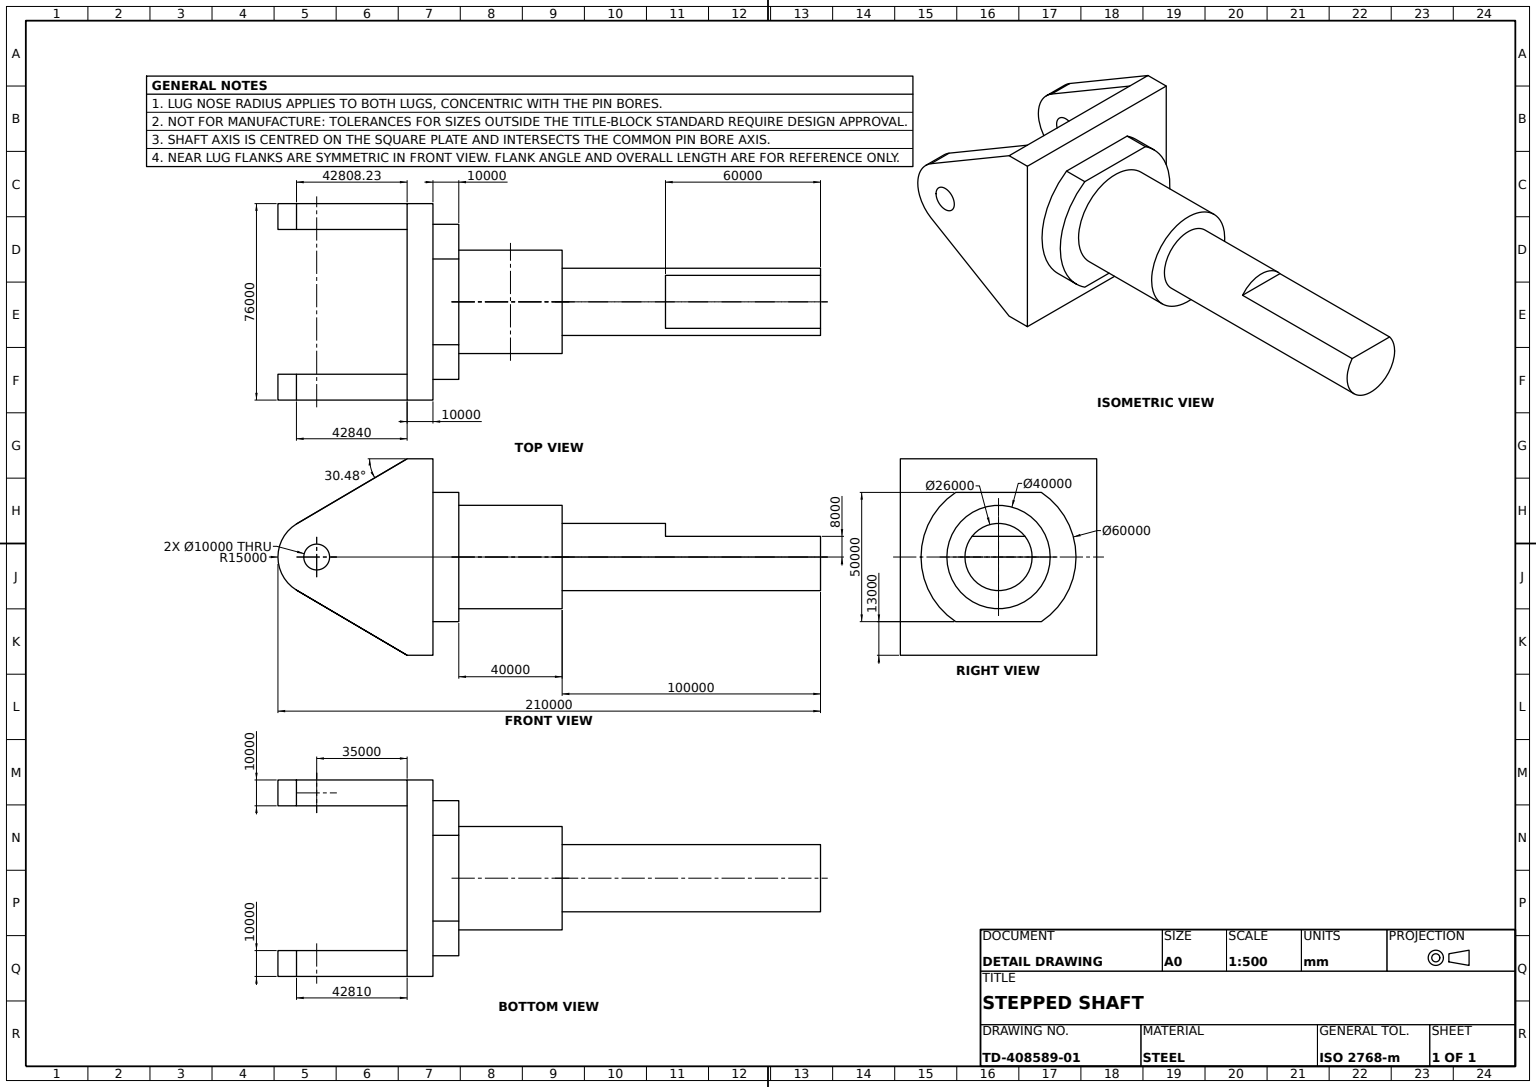
SolidWorks part; units mm, degrees
material "Plain Carbon Steel"
ref_plane "Front Plane" through (0, 0, 0) normal (0, 0, 1) x (1, 0, 0)
ref_plane "Top Plane" through (0, 0, 0) normal (0, 1, 0) x (1, 0, 0)
ref_plane "Right Plane" through (0, 0, 0) normal (1, 0, 0) x (0, 0, -1)
sketch "Base Plate Sketch" plane through (0, 0, 0) normal (0, 0, 1) x (1, 0, 0)
  line L5 (-38000, -38000) -> (38000, -38000)
  line L6 (-38000, -38000) -> (-38000, 38000)
  line L7 (-38000, 38000) -> (38000, 38000)
  line L8 (38000, -38000) -> (38000, 38000)
  line L9 (-38000, -38000) -> (38000, 38000) construction
  line L10 (-38000, 38000) -> (38000, -38000) construction
  point P0 (0, 0)
  dimension "D1" = 38000
extrude "Base Plate" add sketch "Base Plate Sketch" along normal blind 10000
sketch "Clevis Lug A Sketch" plane through (38000, 0, 0) normal (1, 0, 0) x (0, 0, -1)
  line L0 (0, 38000) -> (0, -38000)
  line L1 (0, 0) -> (35000, 0) construction
  line L2 (0, 38000) -> (42808.2335, 12807.4779)
  line L3 (0, -38000) -> (42810, -12806.4007)
  arc A0 (42810, -12806.4007) -> (42405.5538, 13044.4537) centre (35000, 0) ccw
  circle A1 centre (35000, 0) radius 5000
  dimension "D2" = 30000
  dimension "D3" = 10000
  dimension "D1" = 35000
  dimension "D4" = 42808.2335
  dimension "D5" = 42810
extrude "Clevis Lug A" add sketch "Clevis Lug A Sketch" against normal blind 10000
sketch "Clevis Lug B Sketch" plane through (-38000, 0, 0) normal (-1, 0, 0) x (0, 0, 1)
  line L0 (0, 38000) -> (0, -38000)
  line L1 (0, 38000) -> (-42840, 12788.0569)
  line L2 (0, -38000) -> (-42840, -12788.0569)
  circle A0 centre (-35000, 0) radius 5000
  arc A1 (-42840, 12788.0569) -> (-42840, -12788.0569) centre (-35000, 0) ccw
  dimension "D1" = 30000
  dimension "D2" = 10000
  dimension "D3" = 42840
  dimension "D4" = 42840
extrude "Clevis Lug B" add sketch "Clevis Lug B Sketch" against normal blind 10000
sketch "Collar Ø60 Sketch" plane through (0, 0, 10000) normal (0, 0, 1) x (1, 0, 0)
  circle A0 centre (0, 0) radius 30000
  dimension "D1" = 60000
extrude "Collar Ø60" add sketch "Collar Ø60 Sketch" along normal blind 10000
sketch "Hex Collar Cut Sketch" plane through (0, 0, 20000) normal (0, 0, 1) x (1, 0, 0)
  line L1 (-35000, 25000) -> (35000, 25000)
  line L2 (-35000, 25000) -> (-35000, -25000)
  line L3 (-35000, -25000) -> (35000, -25000)
  line L4 (35000, 25000) -> (35000, -25000)
  line L5 (-35000, 25000) -> (35000, -25000) construction
  line L6 (-35000, -25000) -> (35000, 25000) construction
  point P0 (0, 0)
  dimension "D1" = 50000
  dimension "D2" = 70000
extrude "Hex Collar Cut" cut sketch "Hex Collar Cut Sketch" against normal blind 10000 flip side to cut
sketch "Shaft Shoulder Ø40 Sketch" plane through (0, 0, 20000) normal (0, 0, 1) x (1, 0, 0)
  circle A0 centre (0, 0) radius 20000
  dimension "D1" = 40000
extrude "Shaft Shoulder Ø40" add sketch "Shaft Shoulder Ø40 Sketch" along normal blind 40000
sketch "Shaft Ø26 Sketch" plane through (0, 0, 60000) normal (0, 0, 1) x (1, 0, 0)
  circle A0 centre (0, 0) radius 13000
  dimension "D1" = 26000
extrude "Shaft Ø26" add sketch "Shaft Ø26 Sketch" along normal blind 100000
sketch "Shaft Flat Sketch" plane through (0, 0, 160000) normal (0, 0, 1) x (1, 0, 0)
  line L1 (-13341.8036, 8000) -> (13341.8036, 8000)
  line L2 (-13341.8036, 8000) -> (-13341.8036, 18033.0363)
  line L3 (-13341.8036, 18033.0363) -> (13341.8036, 18033.0363)
  line L4 (13341.8036, 8000) -> (13341.8036, 18033.0363)
  line L5 (-13341.8036, 8000) -> (13341.8036, 18033.0363) construction
  line L6 (-13341.8036, 18033.0363) -> (13341.8036, 8000) construction
  point P0 (0, 13016.5182)
  dimension "D1" = 26683.6072
  dimension "D2" = 8000
  dimension "D3" = 10033.0363
  dimension "D4" = 13341.8036
extrude "Shaft Flat Cut" cut sketch "Shaft Flat Sketch" against normal blind 60000
